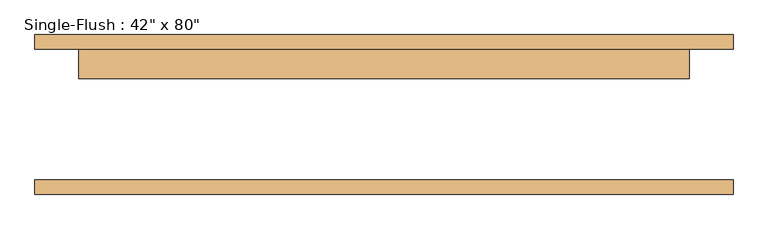
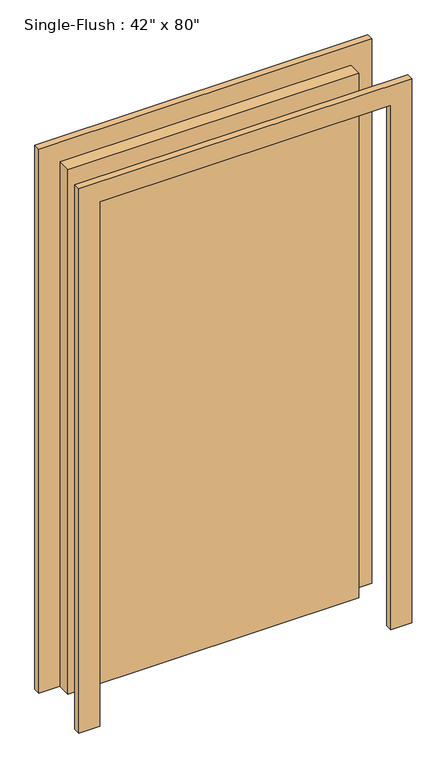
"""IFC4 building model written with IfcOpenShell, lengths in millimetres: door geometry."""

from ifc_helpers import new_model, si_unit, frame, origin, origin_with_axes, place, context, project, spatial, polyline, outline, extrude, source, transform, mapped, element, save


def door_edbf5142(model_context):
    return source(origin(), model_context, "Body", "SweptSolid", [
        extrude(outline(polyline([(2108.2, -609.6), (0.0, -609.6), (0.0, -533.4), (2032.0, -533.4), (2032.0, 533.4), (0.0, 533.4), (0.0, 609.6), (2108.2, 609.6), (2108.2, -609.6)])), frame((0.0, 114.3, 0.0), z_axis=(0.0, 1.0, 0.0), x_axis=(0.0, 0.0, 1.0)), (0.0, 0.0, 1.0), 25.4),
        extrude(outline(polyline([(2108.2, 609.6), (2108.2, -609.6), (0.0, -609.6), (0.0, -533.4), (2032.0, -533.4), (2032.0, 533.4), (0.0, 533.4), (0.0, 609.6), (2108.2, 609.6)])), frame((0.0, -139.7, 0.0), z_axis=(0.0, 1.0, 0.0), x_axis=(0.0, 0.0, 1.0)), (0.0, 0.0, 1.0), 25.4),
        extrude(outline(polyline([(533.4, 63.5), (-533.4, 63.5), (-533.4, 114.3), (533.4, 114.3), (533.4, 63.5)])), origin_with_axes(), (0.0, 0.0, 1.0), 2032.0),
    ])


if __name__ == "__main__":
    model = new_model("IFC4")
    model_context = context("Model", 3, world=origin())
    ifc_project = project(units=[si_unit("LENGTHUNIT", "METRE", prefix="MILLI")], contexts=[model_context])
    site = spatial("IfcSite", under=ifc_project)
    building = spatial("IfcBuilding", under=site)
    placement = place(None, origin())
    door_shape = door_edbf5142(model_context)
    element("IfcDoor", 1, ObjectType="Single-Flush : 42\" x 80\"", at=placement, inside=building, context=model_context, shape_type="MappedRepresentation", body=[
        mapped(door_shape, transform((0.0, 0.0, 0.0), x_axis=(1.0, 0.0, 0.0), y_axis=(0.0, 1.0, 0.0), z_axis=(0.0, 0.0, 1.0))),
    ])
    save(model, "model.ifc")

# Revit data of these elements
# Type "Single-Flush : 42\" x 80\""
#   Type Mark = "15"
#   Construction Type Id = "MDOOR"
#   Assembly Code = "C1020"
#   Analytic Construction = "Metal"
#   Thickness = 0' - 2"
#   Heat Transfer Coefficient (U) = 0.651978 BTU/(h·ft²·°F)
#   Height = 6' - 8"
#   Trim Projection Ext = 0' - 1"
#   Trim Projection Int = 0' - 1"
#   Trim Width = 0' - 3"
#   Width = 3' - 6"
#   Define Thermal Properties by = 1
#   Door Material = Door - Panel
#   Frame Material = Door - Frame
#   Visual Light Transmittance = 0
#   Solar Heat Gain Coefficient = 0
#   Function = (empty or 0)
#   Wall Closure = (empty or 0)
# Element 1 (IfcDoor, "Single-Flush : 42\" x 80\"")
#   Materials on its faces: "Door - Frame", "Door - Panel"
# Materials
#   "Door - Panel": class "Wood", colour RGB 210 159 95, transparency 0, Cost = 0
#   "Door - Frame": colour RGB 118 70 51, transparency 0, Cost = 0
